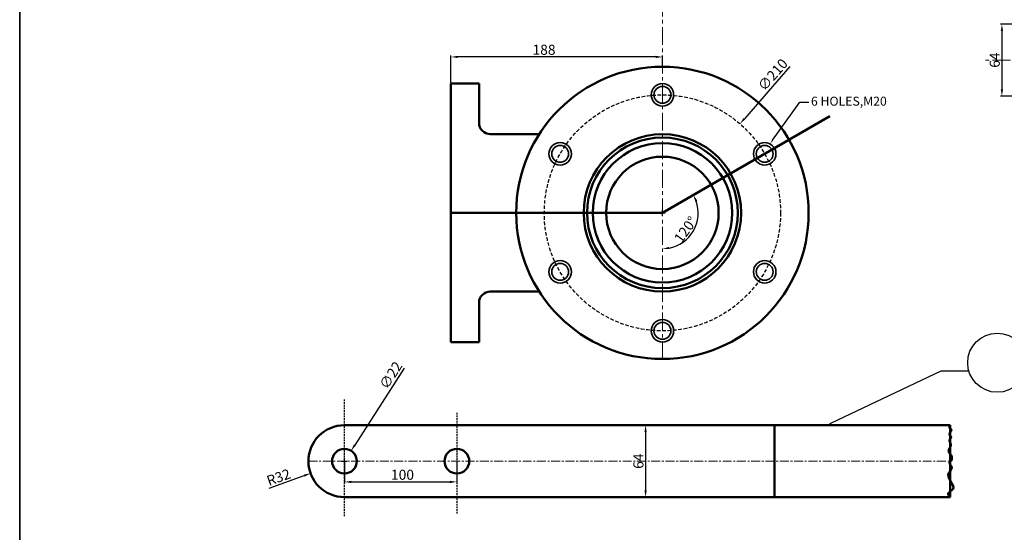
# Model space of a CAD drawing. Units: millimetres. Extents: x -282 to 2335, y -1129 to 664.
# Tile 2 of 8: x -282 to 594, y -368 to 88. Entities that reach past the tile are written whole.
import ezdxf
from ezdxf import colors
from ezdxf.entities.mleader import LeaderData, LeaderLine
from ezdxf.math import Vec2, Vec3

# ---------------------------------------------------------------- set-up
doc = ezdxf.new("R2010")
doc.units = ezdxf.units.MM
doc.header["$LTSCALE"] = 0.5
doc.linetypes.add('CENTER', pattern=[50.8, 31.75, -6.35, 6.35, -6.35])
doc.linetypes.add('HIDDEN', pattern=[9.525, 6.35, -3.175])
for name, color, linetype, lineweight in [('M-CNTR', 1, 'CENTER', 18), ('M-DIMS', 2, 'Continuous', 25), ('M-FAST', 7, 'Continuous', 35), ('M-HIDN', 4, 'HIDDEN', 25), ('M-OUTL', 7, 'Continuous', 50), ('M-TEXT', 3, 'Continuous', 25), ('M-TTLB', 7, 'Continuous', 35)]:
    doc.layers.add(name, color=color, linetype=linetype, lineweight=lineweight)
doc.styles.get("Standard").update_dxf_attribs({"font": 'arial.ttf'})
doc.dimstyles.new('ISO-25', dxfattribs={"dimtxt": 9, "dimasz": 6, "dimexe": 1.25, "dimexo": 0.625, "dimtad": 1, "dimtxsty": 'Standard', "dimcen": 2.5, "dimadec": 0, "dimazin": 0, "dimtfac": 1, "dimtofl": 0, "dimtmove": 0, "dimatfit": 3, "dimfxl": 1, "dimarcsym": 0})

# ---------------------------------------------------------------- blocks, each defined once
blk = doc.blocks.new('*D27')
at = {"layer": 'Defpoints', "color": 0, "transparency": 16777216}
for p in [(358.55, -4.75), (220.73, -163.2)]:
    blk.add_point(p, dxfattribs=at)
at = {"layer": 'M-DIMS', "color": 0, "lineweight": -2, "transparency": 16777216}
for p, q in [((402.89, 46.23), (362.48, -0.22)), ((287.14, -83.98), (292.14, -83.98)), ((289.64, -86.48), (289.64, -81.48))]:
    blk.add_line(p, q, dxfattribs=at)
at = {"layer": 'M-DIMS', "color": 0, "transparency": 16777216}
blk.add_solid([(361.73, 0.43), (363.24, -0.88), (358.55, -4.75)], dxfattribs=at)
at = {"layer": 'M-DIMS', "color": 0, "transparency": 16777216, "insert": (388.62, 38.17), "char_height": 9, "attachment_point": 5, "rotation": 48.98536}
blk.add_mtext('∅210', dxfattribs=at)
blk = doc.blocks.new('*D28')
at = {"layer": 'Defpoints', "color": 0, "transparency": 16777216}
for p in [(101.64, 54.76), (289.64, 46.02), (101.64, 31.02)]:
    blk.add_point(p, dxfattribs=at)
at = {"layer": 'M-DIMS', "color": 0, "lineweight": -2, "transparency": 16777216}
for p, q in [((101.64, 31.65), (101.64, 56.01)), ((283.64, 54.76), (107.64, 54.76)), ((289.64, 46.65), (289.64, 56.01))]:
    blk.add_line(p, q, dxfattribs=at)
at = {"layer": 'M-DIMS', "color": 0, "transparency": 16777216}
for points in [[(107.64, 55.76), (107.64, 53.76), (101.64, 54.76)], [(283.64, 55.76), (283.64, 53.76), (289.64, 54.76)]]:
    blk.add_solid(points, dxfattribs=at)
at = {"layer": 'M-DIMS', "color": 0, "transparency": 16777216, "insert": (184.39, 59.98), "char_height": 9, "attachment_point": 5}
blk.add_mtext('188', dxfattribs=at)
blk = doc.blocks.new('*D29')
at = {"layer": 'Defpoints', "color": 0, "transparency": 16777216}
for p in [(289.64, 408.91), (438.52, 1.98), (289.64, -83.98), (321.01, -89.51), (289.64, -321.19)]:
    blk.add_point(p, dxfattribs=at)
at = {"layer": 'M-DIMS', "color": 0, "lineweight": -2, "transparency": 16777216}
blk.add_arc((289.64, -83.98), 31.85, 280.80805, 19.19195, dxfattribs=at)
at = {"layer": 'M-DIMS', "color": 0, "transparency": 16777216}
for points in [[(318.81, -73.92), (320.63, -73.09), (317.23, -68.05)], [(295.71, -116.26), (295.52, -114.27), (289.64, -115.83)]]:
    blk.add_solid(points, dxfattribs=at)
at = {"layer": 'M-DIMS', "color": 0, "transparency": 16777216, "insert": (311.25, -99.54), "char_height": 9, "attachment_point": 5, "rotation": 54.2496}
blk.add_mtext('120°', dxfattribs=at)
blk = doc.blocks.new('*D46')
at = {"layer": 'Defpoints', "color": 0, "transparency": 16777216}
for p in [(615.29, 83.96), (591.47, 19.96), (615.29, 19.96)]:
    blk.add_point(p, dxfattribs=at)
at = {"layer": 'M-DIMS', "color": 0, "lineweight": -2, "transparency": 16777216}
for p, q in [((614.66, 83.96), (590.22, 83.96)), ((591.47, 77.96), (591.47, 25.96)), ((614.66, 19.96), (590.22, 19.96))]:
    blk.add_line(p, q, dxfattribs=at)
at = {"layer": 'M-DIMS', "color": 0, "transparency": 16777216}
for points in [[(590.47, 77.96), (592.47, 77.96), (591.47, 83.96)], [(590.47, 25.96), (592.47, 25.96), (591.47, 19.96)]]:
    blk.add_solid(points, dxfattribs=at)
at = {"layer": 'M-DIMS', "color": 0, "transparency": 16777216, "insert": (586.25, 51.96), "char_height": 9, "attachment_point": 5, "rotation": 90}
blk.add_mtext('64', dxfattribs=at)
blk = doc.blocks.new('*D98')
at = {"layer": 'Defpoints', "color": 0, "ltscale": 0.5, "transparency": 16777216}
for p in [(6.93, -304.88), (106.93, -304.88), (106.93, -323.34)]:
    blk.add_point(p, dxfattribs=at)
at = {"layer": 'M-DIMS', "color": 0, "lineweight": -2, "ltscale": 0.5, "transparency": 16777216}
for p, q in [((6.93, -305.5), (6.93, -324.59)), ((106.93, -305.5), (106.93, -324.59)), ((12.93, -323.34), (100.93, -323.34))]:
    blk.add_line(p, q, dxfattribs=at)
at = {"layer": 'M-DIMS', "color": 0, "ltscale": 0.5, "transparency": 16777216}
for points in [[(12.93, -322.34), (12.93, -324.34), (6.93, -323.34)], [(100.93, -322.34), (100.93, -324.34), (106.93, -323.34)]]:
    blk.add_solid(points, dxfattribs=at)
at = {"layer": 'M-DIMS', "color": 0, "ltscale": 0.5, "transparency": 16777216, "insert": (58.57, -318.12), "char_height": 9, "attachment_point": 5}
blk.add_mtext('100', dxfattribs=at)
blk = doc.blocks.new('*D103')
at = {"layer": 'Defpoints', "color": 0, "ltscale": 0.5, "transparency": 16777216}
for p in [(12.88, -295.62), (0.99, -314.13)]:
    blk.add_point(p, dxfattribs=at)
at = {"layer": 'M-DIMS', "color": 0, "lineweight": -2, "ltscale": 0.5, "transparency": 16777216}
for p, q in [((60.18, -221.99), (16.12, -290.57)), ((4.43, -304.88), (9.43, -304.88)), ((6.93, -307.38), (6.93, -302.38))]:
    blk.add_line(p, q, dxfattribs=at)
at = {"layer": 'M-DIMS', "color": 0, "ltscale": 0.5, "transparency": 16777216}
blk.add_solid([(15.28, -290.03), (16.96, -291.12), (12.88, -295.62)], dxfattribs=at)
at = {"layer": 'M-DIMS', "color": 0, "ltscale": 0.5, "transparency": 16777216, "insert": (49.14, -229.06), "char_height": 9, "attachment_point": 5, "rotation": 57.28114}
blk.add_mtext('∅22', dxfattribs=at)
blk = doc.blocks.new('*D104')
at = {"layer": 'Defpoints', "color": 0, "ltscale": 0.5, "transparency": 16777216}
for p in [(6.93, -304.88), (-23.18, -315.71)]:
    blk.add_point(p, dxfattribs=at)
at = {"layer": 'M-DIMS', "color": 0, "lineweight": -2, "ltscale": 0.5, "transparency": 16777216}
for p, q in [((4.43, -304.88), (9.43, -304.88)), ((6.93, -307.38), (6.93, -302.38)), ((-60.11, -329), (-28.82, -317.74))]:
    blk.add_line(p, q, dxfattribs=at)
at = {"layer": 'M-DIMS', "color": 0, "ltscale": 0.5, "transparency": 16777216}
blk.add_solid([(-29.16, -316.8), (-28.48, -318.69), (-23.18, -315.71)], dxfattribs=at)
at = {"layer": 'M-DIMS', "color": 0, "ltscale": 0.5, "transparency": 16777216, "insert": (-51.22, -320.25), "char_height": 9, "attachment_point": 5, "rotation": 19.7915}
blk.add_mtext('R32', dxfattribs=at)
blk = doc.blocks.new('*D105')
at = {"layer": 'Defpoints', "color": 0, "ltscale": 0.5, "transparency": 16777216}
for p in [(304.41, -272.88), (274.66, -336.88), (304.41, -336.88)]:
    blk.add_point(p, dxfattribs=at)
at = {"layer": 'M-DIMS', "color": 0, "lineweight": -2, "ltscale": 0.5, "transparency": 16777216}
for p, q in [((303.78, -272.88), (273.41, -272.88)), ((274.66, -278.88), (274.66, -330.88)), ((303.78, -336.88), (273.41, -336.88))]:
    blk.add_line(p, q, dxfattribs=at)
at = {"layer": 'M-DIMS', "color": 0, "ltscale": 0.5, "transparency": 16777216}
for points in [[(273.66, -278.88), (275.66, -278.88), (274.66, -272.88)], [(273.66, -330.88), (275.66, -330.88), (274.66, -336.88)]]:
    blk.add_solid(points, dxfattribs=at)
at = {"layer": 'M-DIMS', "color": 0, "ltscale": 0.5, "transparency": 16777216, "insert": (269.44, -304.88), "char_height": 9, "attachment_point": 5, "rotation": 90}
blk.add_mtext('64', dxfattribs=at)
blk = doc.blocks.new('STUD-M20')
for radius in [10, 7.5]:
    blk.add_circle((10, 10), radius)

msp = doc.modelspace()

# ---------------------------------------------------------------- linework, layer by layer
at = {"layer": 'M-CNTR'}
for p, q in [((289.639, -213.977), (289.639, 408.911)), ((903.869, 51.958), (576.271, 51.958))]:
    msp.add_line(p, q, dxfattribs=at)
at = {"layer": 'M-CNTR', "ltscale": 0.5}
msp.add_line((-25.067, -304.877), (545.504, -304.877), dxfattribs=at)
at = {"layer": 'M-HIDN', "ltscale": 0.5}
for p, q in [((6.933, -353.878), (6.933, -249.126)), ((106.933, -261.803), (106.933, -352.2))]:
    msp.add_line(p, q, dxfattribs=at)
at = {"layer": 'M-HIDN'}
msp.add_circle((289.639, -83.977), 105, dxfattribs=at)
at = {"layer": 'M-OUTL'}
for p, q in [((101.639, -198.977), (101.639, 31.023)), ((126.639, 31.023), (101.639, 31.023)), ((126.639, -3.977), (126.639, 31.023)), ((289.639, -83.977), (438.52, 1.98)), ((180.094, -13.977), (136.639, -13.977)), ((289.639, -83.977), (101.639, -83.977)), ((180.094, -153.977), (136.639, -153.977)), ((126.639, -198.977), (126.639, -163.977)), ((101.639, -198.977), (126.639, -198.977))]:
    msp.add_line(p, q, dxfattribs=at)
at = {"layer": 'M-OUTL', "ltscale": 0.5}
for p, q in [((6.933, -272.877), (545.504, -272.877)), ((389.424, -272.877), (389.424, -336.877)), ((545.504, -272.877), (545.504, -336.877)), ((6.933, -336.877), (545.504, -336.877))]:
    msp.add_line(p, q, dxfattribs=at)
at = {"layer": 'M-OUTL'}
for radius in [130, 70, 67, 62, 50]:
    msp.add_circle((289.639, -83.977), radius, dxfattribs=at)
at = {"layer": 'M-OUTL', "ltscale": 0.5}
for centre in [(6.933, -304.877), (106.933, -304.877)]:
    msp.add_circle(centre, 11, dxfattribs=at)
at = {"layer": 'M-OUTL'}
for centre, start, end in [((136.639, -3.977), 180, 270), ((136.639, -163.977), 90, 180)]:
    msp.add_arc(centre, 10, start, end, dxfattribs=at)
at = {"layer": 'M-OUTL', "ltscale": 0.5}
msp.add_arc((6.933, -304.877), 32, 90, 270, dxfattribs=at)
msp.add_open_spline([(545.504, -272.877), (545.02, -273.67), (544.047, -275.264), (547.388, -276.617), (545.488, -279.135), (543.891, -281.701), (547.763, -283.324), (543.434, -286.562), (547.144, -289.876), (544.668, -293.084), (543.547, -296.919), (547.051, -299.554), (547.58, -304.042), (543.445, -306.346), (549.451, -310.605), (542.282, -315.42), (545.156, -322.454), (551.122, -329.734), (541.752, -333.127), (544.525, -335.899), (545.504, -336.877)], degree=3, knots=[0, 0, 0, 0, 2.3007615, 4.6275372, 7.2843318, 9.7954463, 12.058629, 15.7220618, 19.241454, 22.866589, 26.3168237, 29.9012252, 34.8289121, 36.8244164, 41.4125925, 47.5020067, 54.4341763, 62.2769446, 68.5666149, 71.9941067, 71.9941067, 71.9941067, 71.9941067], dxfattribs=at)
at = {"layer": 'M-TEXT'}
msp.add_circle((587.312, -217.331), 26.287, dxfattribs=at)
at = {"layer": 'M-TTLB', "ltscale": 0.5}
msp.add_lwpolyline([(-281.776, 663.767), (2334.915, 663.767), (2334.915, -1128.523), (-281.776, -1128.523)], close=True, dxfattribs=at)

# ---------------------------------------------------------------- block references
at = {"layer": 'M-FAST'}
for p in [(279.638, 11.023), (188.706, -41.477), (370.571, -41.477), (188.706, -146.477), (370.571, -146.477), (279.638, -198.977)]:
    msp.add_blockref('STUD-M20', p, dxfattribs=at)

# ---------------------------------------------------------------- dimensions: what is measured, and where the dimension line sits
at = {"layer": 'M-DIMS'}
dim = msp.add_angular_dim_2l(base=(321.009, -89.508), line1=((289.639, -83.977), (438.52, 1.98)), line2=((289.639, -321.193), (289.639, 408.911)), dimstyle='ISO-25', override={"dimclrd": 0, "dimclre": 0, "dimclrt": 0}, dxfattribs=at)
dim.commit()
dim.dimension.update_dxf_attribs({"geometry": '*D29', "text_midpoint": (315.491, -102.588), "dimtype": 162})
dim = msp.add_linear_dim(base=(591.474, 19.958), p1=(615.287, 83.958), p2=(615.287, 19.958), angle=90, dimstyle='ISO-25', override={"dimclrd": 0, "dimclre": 0, "dimclrt": 0}, dxfattribs=at)
dim.commit()
dim.dimension.update_dxf_attribs({"geometry": '*D46', "text_midpoint": (591.474, 51.958), "dimtype": 160})
dim = msp.add_linear_dim(base=(101.639, 54.764), p1=(289.639, 46.023), p2=(101.639, 31.023), dimstyle='ISO-25', override={"dimclrd": 0, "dimclre": 0, "dimclrt": 0}, dxfattribs=at)
dim.commit()
dim.dimension.update_dxf_attribs({"geometry": '*D28', "text_midpoint": (184.389, 54.764), "dimtype": 160})
dim = msp.add_diameter_dim_2p(p1=(220.732, -163.204), p2=(358.545, -4.75), dimstyle='ISO-25', override={"dimclrd": 0, "dimclre": 0, "dimclrt": 0}, dxfattribs=at)
dim.commit()
dim.dimension.update_dxf_attribs({"geometry": '*D27', "text_midpoint": (392.747, 34.575), "dimtype": 163})
at = {"layer": 'M-DIMS', "ltscale": 0.5}
dim = msp.add_diameter_dim_2p(p1=(0.987, -314.132), p2=(12.879, -295.623), dimstyle='ISO-25', override={"dimclrd": 0, "dimclre": 0, "dimclrt": 0}, dxfattribs=at)
dim.commit()
dim.dimension.update_dxf_attribs({"geometry": '*D103', "text_midpoint": (53.74, -232.021), "dimtype": 163})
dim = msp.add_linear_dim(base=(274.658, -336.877), p1=(304.407, -272.877), p2=(304.407, -336.877), angle=90, dimstyle='ISO-25', override={"dimclrd": 0, "dimclre": 0, "dimclrt": 0}, dxfattribs=at)
dim.commit()
dim.dimension.update_dxf_attribs({"geometry": '*D105', "text_midpoint": (274.658, -304.877), "dimtype": 160})
dim = msp.add_radius_dim(center=(6.933, -304.877), mpoint=(-23.177, -315.713), dimstyle='ISO-25', override={"dimclrd": 0, "dimclre": 0, "dimclrt": 0}, dxfattribs=at)
dim.commit()
dim.dimension.update_dxf_attribs({"geometry": '*D104', "text_midpoint": (-49.45, -325.167), "dimtype": 164})
dim = msp.add_linear_dim(base=(106.933, -323.335), p1=(6.933, -304.877), p2=(106.933, -304.877), dimstyle='ISO-25', override={"dimclrd": 0, "dimclre": 0, "dimclrt": 0}, dxfattribs=at)
dim.commit()
dim.dimension.update_dxf_attribs({"geometry": '*D98', "text_midpoint": (58.566, -323.335), "dimtype": 160})

# ---------------------------------------------------------------- leaders
at = {"layer": 'M-TEXT'}
ml = msp.add_multileader_mtext('Standard', dxfattribs=at)
ml.set_content('6 HOLES DIA 20', color=256)
ml.set_leader_properties()
ml.build(insert=Vec2(0, 0))
ctx = ml.context
ctx.base_point, ctx.char_height, ctx.plane_origin = Vec3(27.18, 100.339), 8, Vec3(199.639, 130.844)
ctx.text_align_type = 2
notes = []
notes.append((ctx, [(0, (1, 1, 0), (122.706, 100.339), (-1, 0), 8, [(0, [(199.639, 130.844)], 0, [])])]))
ctx.mtext.insert, ctx.mtext.alignment, ctx.mtext.flow_direction = Vec3(112.706, 104.407), 3, 5
ml = msp.add_multileader_mtext('Standard', dxfattribs=at)
ml.set_content('6 HOLES,M20', color=256)
ml.set_leader_properties()
ml.build(insert=Vec2(0, 0))
ctx = ml.context
ctx.base_point, ctx.char_height, ctx.plane_origin = Vec3(419.714, 14.59), 8, Vec3(385.295, -22.663)
notes.append((ctx, [(0, (1, 1, 0), (411.714, 14.59), (1, 0), 8, [(0, [(385.295, -22.663)], 0, [])])]))
ctx.mtext.insert, ctx.mtext.flow_direction = Vec3(421.714, 19.381), 5
at = {"layer": 'M-TEXT', "ltscale": 0.5}
ml = msp.add_multileader_mtext('Standard', dxfattribs=at)
ml.set_content('', color=256)
ml.set_leader_properties()
ml.build(insert=Vec2(0, 0))
ctx = ml.context
ctx.base_point, ctx.plane_origin = Vec3(561.999, -224.418), Vec3(435.879, -272.877)
notes.append((ctx, [(0, (1, 1, 0), (537.562, -224.418), (1, 0), 24.437, [(0, [(435.879, -272.877)], 0, [])])]))
ctx.mtext.insert, ctx.mtext.flow_direction = Vec3(563.999, -222.418), 5
for ctx, leaders in notes:
    for number, flags, end, landing, length, lines in leaders:
        leader = LeaderData()
        leader.index, (leader.has_last_leader_line, leader.has_dogleg_vector, leader.attachment_direction) = number, flags
        leader.last_leader_point, leader.dogleg_vector, leader.dogleg_length = Vec3(end), Vec3(landing), length
        for number, points, colour, breaks in lines:
            line = LeaderLine()
            line.index, line.vertices, line.color, line.breaks = number, Vec3.list(points), colors.encode_raw_color(colour), breaks
            leader.lines.append(line)
        ctx.leaders.append(leader)

doc.saveas('drawing.dxf')
